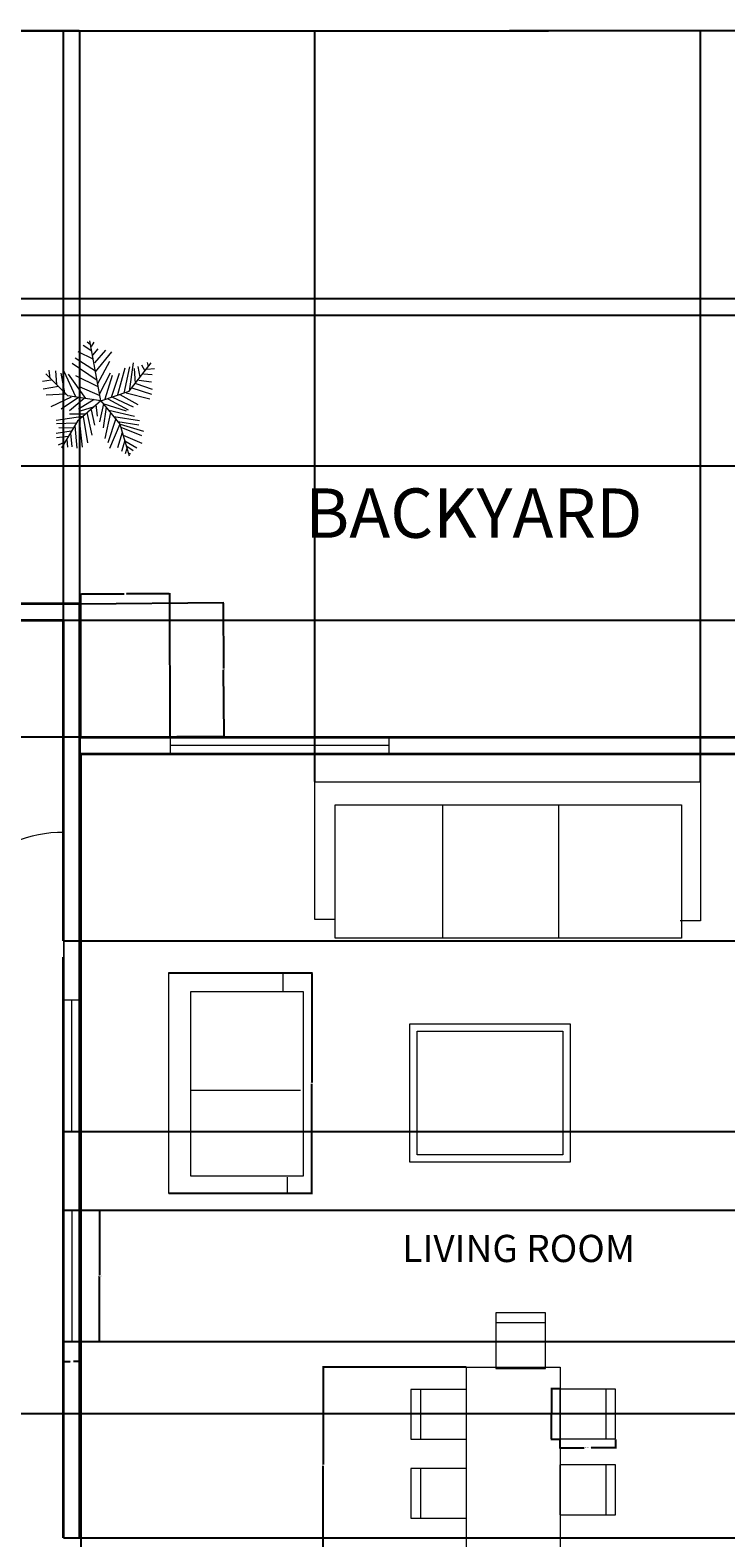
# Model space of a CAD drawing. Units: inches. Extents: x -86 to 773, y -188 to 560.
# Tile 3 of 6: x 201 to 392, y 147 to 560. Entities that reach past the tile are written whole.
import ezdxf

# ---------------------------------------------------------------- set-up
doc = ezdxf.new("R2010")
doc.units = ezdxf.units.IN
doc.header["$MEASUREMENT"] = 0
for name, color, linetype, lineweight in [('A-ANNO-DIMS', 2, 'Continuous', 18), ('A-AREA-IDEN', 7, 'Continuous', 25), ('A-DOOR', 7, 'Continuous', 18), ('A-FURN', 8, 'Continuous', 18), ('A-GLAZ', 7, 'Continuous', 18), ('A-WALL', 7, 'Continuous', 35), ('C-PROP', 7, 'Continuous', 25), ('L-PLNT-TREE', 8, 'Continuous', 9)]:
    doc.layers.add(name, color=color, linetype=linetype, lineweight=lineweight)
doc.styles.get("Standard").update_dxf_attribs({"font": 'arial.ttf'})
doc.dimstyles.get("Standard").update_dxf_attribs({"dimtxt": 0.18, "dimasz": 0.18, "dimexe": 0.18, "dimexo": 0.0625, "dimgap": 0.09, "dimtad": 0, "dimtih": 1, "dimtoh": 1, "dimdec": 4, "dimzin": 0, "dimdsep": 46, "dimtxsty": 'Standard', "dimcen": 0.09, "dimadec": 0, "dimazin": 0, "dimtfac": 1, "dimtdec": 4, "dimtofl": 0, "dimtmove": 0, "dimatfit": 3, "dimfxl": 1, "dimtolj": 1, "dimtzin": 0, "dimarcsym": 0})

# ---------------------------------------------------------------- blocks, each defined once
blk = doc.blocks.new('Trees - Metric')
for p, q in [((-185.1152, 1008.5578), (-553.1612, 1185.4942)), ((-221.9198, 1197.3052), (-433.5526, 1338.8594)), ((-258.7244, 1362.456), (-332.3336, 1421.4348)), ((0, 0), (-266.7, 1447.8)), ((-231.1146, 1315.2628), (-166.7002, 1421.4348)), ((-194.31, 1102.9442), (-65.4812, 1256.284)), ((-148.3106, 914.1968), (118.5418, 1220.9018)), ((-129.8956, 701.8528), (265.7602, 1185.4942)), ((-1234.059, 536.7274), (-1252.4486, 737.2604)), ((-93.091, 489.5342), (-700.3796, 902.3858)), ((-129.8956, 713.6638), (-626.7704, 1032.1544)), ((-74.7014, 418.7444), (219.7608, 961.39)), ((412.9786, 147.447), (587.8068, 796.2392)), ((560.197, 182.8292), (698.2206, 819.8358)), ((685.8, 228.6), (1219.2, 914.4)), ((689.0258, 230.0224), (790.2448, 914.1968)), ((808.6344, 784.4282), (827.0494, 418.7444)), ((891.4384, 831.6214), (946.658, 572.1096)), ((983.4626, 867.0036), (1066.2666, 725.4494)), ((1112.2914, 760.8316), (1296.3144, 784.4282)), ((1121.4862, 925.9824), (1149.0706, 831.6214)), ((-1206.4492, 501.3198), (-1418.082, 465.9376)), ((-800.1, 114.3), (-1333.5, 647.7)), ((-1105.2302, 725.4494), (-1077.6458, 395.1732)), ((-976.4268, 666.4706), (-884.4026, 194.6402)), ((-902.8176, 713.6638), (-617.5756, 100.2538)), ((-369.1382, 53.086), (-783.1836, 642.874)), ((-617.5756, 607.4918), (-74.7014, 347.98)), ((-28.6766, 171.0436), (228.9556, 678.2816)), ((100.1268, 41.275), (284.1498, 619.2774)), ((256.5654, 88.4682), (449.7832, 666.4706)), ((845.439, 418.7444), (1241.0948, 277.1902)), ((919.0482, 501.3198), (1222.6798, 454.152)), ((1029.462, 654.685), (1241.0948, 631.0884)), ((-1031.621, 347.98), (-1399.667, 277.1902)), ((-847.598, 159.2326), (-1326.0578, 135.636)), ((-718.7946, 88.4682), (-1215.644, -147.447)), ((-543.9664, 76.6572), (-967.2066, -206.4512)), ((0, 0), (-800.1, 114.3)), ((-405.9428, 53.086), (-764.794, -241.8334)), ((0, 0), (-571.5, -495.3)), ((-166.7002, 29.4894), (-543.9664, -206.4512)), ((-525.5514, 347.98), (-28.6766, 123.8504)), ((0, 0), (685.8, 228.6)), ((0, 0), (457.2, -571.5)), ((164.5412, 41.275), (661.416, -218.2368)), ((284.1498, 88.4682), (781.0246, -147.447)), ((458.978, 147.447), (891.4384, -88.4682)), ((615.4166, 194.6402), (1185.8752, 41.275)), ((753.4148, 312.5978), (1222.6798, 159.2326)), ((-387.5278, -324.4088), (-764.794, -324.4088)), ((-166.7002, -147.447), (-507.1618, -253.619)), ((-341.5284, -289.0012), (-221.9198, -831.6214)), ((-240.3094, -218.2368), (-157.5054, -595.7062)), ((-120.7008, -88.4682), (-93.091, -371.5766)), ((63.3222, -76.6826), (-37.8714, -513.1308)), ((44.9326, -64.897), (615.4166, -241.8334)), ((127.7366, -159.258), (54.1274, -654.685)), ((228.9556, -289.0012), (90.932, -914.1968)), ((192.151, -230.0224), (817.8292, -371.5766)), ((-442.7474, -383.3876), (-1086.8406, -477.7486)), ((-617.5756, -548.5384), (-1077.6458, -560.324)), ((-681.9646, -666.496), (-1022.4262, -654.685)), ((-571.5, -495.3), (-952.5, -1143)), ((-635.9652, -607.5172), (-580.771, -1150.1374)), ((-525.5514, -465.963), (-451.9422, -1126.5408)), ((-433.5526, -383.3876), (-323.1134, -1020.3688)), ((357.759, -430.5554), (164.5412, -1020.3688)), ((458.978, -572.1096), (210.5406, -1161.923)), ((311.7596, -383.3876), (937.4378, -477.7486)), ((412.9786, -501.3452), (919.0482, -583.9206)), ((457.2, -571.5), (685.8, -1333.5)), ((468.1982, -572.1096), (1029.462, -737.2604)), ((486.5878, -642.8994), (983.4626, -843.4324)), ((-718.7946, -737.2604), (-1086.8406, -796.2392)), ((-783.1836, -867.029), (-1077.6458, -902.4112)), ((-875.2078, -1008.5832), (-1040.8412, -1079.3476)), ((-829.2084, -937.7934), (-810.7934, -1126.5408)), ((-737.1842, -784.4536), (-709.5744, -1114.7298)), ((514.1976, -772.6426), (403.7838, -1138.3264)), ((578.612, -961.39), (495.7826, -1232.7128)), ((541.8074, -831.6214), (992.6574, -1032.1544)), ((578.612, -973.1756), (873.0488, -1138.3264)), ((624.6114, -1161.923), (587.8068, -1291.6916)), ((624.6114, -1102.9442), (781.0246, -1209.1162)), ((679.8056, -1268.095), (716.6102, -1291.6916))]:
    blk.add_line(p, q)
blk = doc.blocks.new('WIN-60-W4_5')
for p, q in [((0, 4.5), (0, 0)), ((60, 4.5), (60, 0)), ((60, 2.25), (0, 2.25))]:
    blk.add_line(p, q)
blk = doc.blocks.new('WIN-36-W4_5')
for p, q in [((0, 36), (4.5, 36)), ((2.25, 36), (2.25, 0)), ((0, 0), (4.5, 0))]:
    blk.add_line(p, q)
blk = doc.blocks.new('DINING-CHAIR')
blk.add_line((0, 12.55), (13.8, 12.55))
blk.add_lwpolyline([(0.02, 0), (13.65, 0), (13.65, 15.22), (0.02, 15.22)], close=True)
blk = doc.blocks.new('*D19')
at = {"layer": 'A-ANNO-DIMS', "color": 0, "lineweight": -2, "transparency": 16777216}
for p, q in [((346.32, 174.18), (346.32, 171.78)), ((361.54, 174.18), (361.54, 171.78)), ((346.5, 171.96), (352.98, 171.96)), ((361.36, 171.96), (354.89, 171.96))]:
    blk.add_line(p, q, dxfattribs=at)
at = {"layer": 'A-ANNO-DIMS', "color": 0, "transparency": 16777216}
for points in [[(346.5, 171.99), (346.5, 171.93), (346.32, 171.96)], [(361.36, 171.99), (361.36, 171.93), (361.54, 171.96)]]:
    blk.add_solid(points, dxfattribs=at)
at = {"layer": 'Defpoints', "color": 0, "transparency": 16777216}
for p in [(346.32, 174.25), (361.54, 174.25), (361.54, 171.96)]:
    blk.add_point(p, dxfattribs=at)
at = {"layer": 'A-ANNO-DIMS', "color": 0, "transparency": 16777216, "insert": (353.93, 171.96), "char_height": 0.18, "attachment_point": 5}
blk.add_mtext('\\A1;CHAIR 15 TYP.', dxfattribs=at)
blk = doc.blocks.new('*D20')
at = {"layer": 'A-ANNO-DIMS', "color": 0, "lineweight": -2, "transparency": 16777216}
for p, q in [((346.26, 188.05), (343.86, 188.05)), ((344.04, 187.87), (344.04, 181.33)), ((344.04, 174.43), (344.04, 180.97)), ((346.26, 174.25), (343.86, 174.25))]:
    blk.add_line(p, q, dxfattribs=at)
at = {"layer": 'A-ANNO-DIMS', "color": 0, "transparency": 16777216}
for points in [[(344.01, 187.87), (344.07, 187.87), (344.04, 188.05)], [(344.01, 174.43), (344.07, 174.43), (344.04, 174.25)]]:
    blk.add_solid(points, dxfattribs=at)
at = {"layer": 'Defpoints', "color": 0, "transparency": 16777216}
for p in [(346.32, 188.05), (344.04, 174.25), (346.32, 174.25)]:
    blk.add_point(p, dxfattribs=at)
at = {"layer": 'A-ANNO-DIMS', "color": 0, "transparency": 16777216, "insert": (344.04, 181.15), "char_height": 0.18, "attachment_point": 5}
blk.add_mtext('\\A1;14 TYP.', dxfattribs=at)
blk = doc.blocks.new('*D37')
at = {"layer": 'A-ANNO-DIMS', "color": 0, "lineweight": -2, "transparency": 16777216}
for p, q in [((214.83, 237.01), (220.34, 237.01)), ((220.16, 236.83), (220.16, 219.19)), ((220.16, 201.19), (220.16, 218.82)), ((214.83, 201.01), (220.34, 201.01))]:
    blk.add_line(p, q, dxfattribs=at)
at = {"layer": 'A-ANNO-DIMS', "color": 0, "transparency": 16777216}
for points in [[(220.13, 236.83), (220.19, 236.83), (220.16, 237.01)], [(220.13, 201.19), (220.19, 201.19), (220.16, 201.01)]]:
    blk.add_solid(points, dxfattribs=at)
at = {"layer": 'Defpoints', "color": 0, "transparency": 16777216}
for p in [(214.76, 237.01), (220.16, 237.01), (214.76, 201.01)]:
    blk.add_point(p, dxfattribs=at)
at = {"layer": 'A-ANNO-DIMS', "color": 0, "transparency": 16777216, "insert": (220.16, 219.01), "char_height": 0.18, "attachment_point": 5}
blk.add_mtext('\\A1;WINDOW 36 TYP.', dxfattribs=at)
blk = doc.blocks.new('*D38')
at = {"layer": 'A-ANNO-DIMS', "color": 0, "lineweight": -2, "transparency": 16777216}
for p, q in [((210.26, 200.94), (210.26, 195.43)), ((214.76, 200.94), (214.76, 195.43)), ((210.44, 195.61), (212.06, 195.61)), ((214.58, 195.61), (212.97, 195.61))]:
    blk.add_line(p, q, dxfattribs=at)
at = {"layer": 'A-ANNO-DIMS', "color": 0, "transparency": 16777216}
for points in [[(210.44, 195.64), (210.44, 195.58), (210.26, 195.61)], [(214.58, 195.64), (214.58, 195.58), (214.76, 195.61)]]:
    blk.add_solid(points, dxfattribs=at)
at = {"layer": 'Defpoints', "color": 0, "transparency": 16777216}
for p in [(210.26, 201.01), (214.76, 201.01), (214.76, 195.61)]:
    blk.add_point(p, dxfattribs=at)
at = {"layer": 'A-ANNO-DIMS', "color": 0, "transparency": 16777216, "insert": (212.51, 195.61), "char_height": 0.18, "attachment_point": 5}
blk.add_mtext('\\A1;5 TYP.', dxfattribs=at)
blk = doc.blocks.new('*D45')
at = {"layer": 'A-ANNO-DIMS', "color": 0, "lineweight": -2, "transparency": 16777216}
for p, q in [((-46.55, 486.72), (-46.55, 560.19)), ((-46.37, 560.01), (343.16, 560.01)), ((733.27, 560.01), (343.74, 560.01)), ((733.45, 486.72), (733.45, 560.19))]:
    blk.add_line(p, q, dxfattribs=at)
at = {"layer": 'A-ANNO-DIMS', "color": 0, "transparency": 16777216}
for points in [[(-46.37, 560.04), (-46.37, 559.98), (-46.55, 560.01)], [(733.27, 560.04), (733.27, 559.98), (733.45, 560.01)]]:
    blk.add_solid(points, dxfattribs=at)
at = {"layer": 'Defpoints', "color": 0, "transparency": 16777216}
for p in [(733.45, 560.01), (-46.55, 486.66), (733.45, 486.66)]:
    blk.add_point(p, dxfattribs=at)
at = {"layer": 'A-ANNO-DIMS', "color": 0, "transparency": 16777216, "insert": (343.45, 560.01), "char_height": 0.18, "attachment_point": 5}
blk.add_mtext('\\A1;780', dxfattribs=at)
blk = doc.blocks.new('*D55')
at = {"layer": 'A-ANNO-DIMS', "color": 0, "lineweight": -2, "transparency": 16777216}
for p, q in [((450.97, 440.74), (-85.98, 440.74)), ((-85.8, 440.56), (-85.8, 403.81)), ((-85.8, 366.7), (-85.8, 403.45)), ((450.97, 366.52), (-85.98, 366.52))]:
    blk.add_line(p, q, dxfattribs=at)
at = {"layer": 'A-ANNO-DIMS', "color": 0, "transparency": 16777216}
for points in [[(-85.83, 440.56), (-85.77, 440.56), (-85.8, 440.74)], [(-85.83, 366.7), (-85.77, 366.7), (-85.8, 366.52)]]:
    blk.add_solid(points, dxfattribs=at)
at = {"layer": 'Defpoints', "color": 0, "transparency": 16777216}
for p in [(451.03, 440.74), (-85.8, 366.52), (451.03, 366.52)]:
    blk.add_point(p, dxfattribs=at)
at = {"layer": 'A-ANNO-DIMS', "color": 0, "transparency": 16777216, "insert": (-85.8, 403.63), "char_height": 0.18, "attachment_point": 5}
blk.add_mtext('\\A1;74.22', dxfattribs=at)
blk = doc.blocks.new('*D56')
at = {"layer": 'A-ANNO-DIMS', "color": 0, "lineweight": -2, "transparency": 16777216}
for p, q in [((13.45, 403.19), (13.45, 560.19)), ((13.63, 560.01), (113.71, 560.01)), ((214.57, 560.01), (114.5, 560.01)), ((214.75, 403.19), (214.75, 560.19))]:
    blk.add_line(p, q, dxfattribs=at)
at = {"layer": 'A-ANNO-DIMS', "color": 0, "transparency": 16777216}
for points in [[(13.63, 560.04), (13.63, 559.98), (13.45, 560.01)], [(214.57, 560.04), (214.57, 559.98), (214.75, 560.01)]]:
    blk.add_solid(points, dxfattribs=at)
at = {"layer": 'Defpoints', "color": 0, "transparency": 16777216}
for p in [(214.75, 560.01), (13.45, 403.12), (214.75, 403.12)]:
    blk.add_point(p, dxfattribs=at)
at = {"layer": 'A-ANNO-DIMS', "color": 0, "transparency": 16777216, "insert": (114.1, 560.01), "char_height": 0.18, "attachment_point": 5}
blk.add_mtext('\\A1;201.3', dxfattribs=at)
blk = doc.blocks.new('*D58')
at = {"layer": 'A-ANNO-DIMS', "color": 0, "lineweight": -2, "transparency": 16777216}
for p, q in [((136.03, 398.69), (136.03, 560.19)), ((136.21, 560.01), (172.75, 560.01)), ((210.07, 560.01), (173.53, 560.01)), ((210.25, 398.69), (210.25, 560.19))]:
    blk.add_line(p, q, dxfattribs=at)
at = {"layer": 'A-ANNO-DIMS', "color": 0, "transparency": 16777216}
for points in [[(136.21, 560.04), (136.21, 559.98), (136.03, 560.01)], [(210.07, 560.04), (210.07, 559.98), (210.25, 560.01)]]:
    blk.add_solid(points, dxfattribs=at)
at = {"layer": 'Defpoints', "color": 0, "transparency": 16777216}
for p in [(210.25, 560.01), (136.03, 398.62), (210.25, 398.62)]:
    blk.add_point(p, dxfattribs=at)
at = {"layer": 'A-ANNO-DIMS', "color": 0, "transparency": 16777216, "insert": (173.14, 560.01), "char_height": 0.18, "attachment_point": 5}
blk.add_mtext('\\A1;74.22', dxfattribs=at)
blk = doc.blocks.new('*D61')
at = {"layer": 'A-ANNO-DIMS', "color": 0, "lineweight": -2, "transparency": 16777216}
for p, q in [((210.31, 398.62), (772.88, 398.62)), ((772.7, 398.44), (772.7, 354.88)), ((772.7, 310.95), (772.7, 354.52)), ((210.31, 310.77), (772.88, 310.77))]:
    blk.add_line(p, q, dxfattribs=at)
at = {"layer": 'A-ANNO-DIMS', "color": 0, "transparency": 16777216}
for points in [[(772.67, 398.44), (772.73, 398.44), (772.7, 398.62)], [(772.67, 310.95), (772.73, 310.95), (772.7, 310.77)]]:
    blk.add_solid(points, dxfattribs=at)
at = {"layer": 'Defpoints', "color": 0, "transparency": 16777216}
for p in [(210.25, 398.62), (210.25, 310.77), (772.7, 310.77)]:
    blk.add_point(p, dxfattribs=at)
at = {"layer": 'A-ANNO-DIMS', "color": 0, "transparency": 16777216, "insert": (772.7, 354.7), "char_height": 0.18, "attachment_point": 5}
blk.add_mtext('\\A1;87.85', dxfattribs=at)
blk = doc.blocks.new('*D62')
at = {"layer": 'A-ANNO-DIMS', "color": 0, "lineweight": -2, "transparency": 16777216}
for p, q in [((210.33, 201.01), (772.88, 201.01)), ((772.7, 200.83), (772.7, 174.33)), ((772.7, 147.46), (772.7, 173.96)), ((210.31, 147.28), (772.88, 147.28))]:
    blk.add_line(p, q, dxfattribs=at)
at = {"layer": 'A-ANNO-DIMS', "color": 0, "transparency": 16777216}
for points in [[(772.67, 200.83), (772.73, 200.83), (772.7, 201.01)], [(772.67, 147.46), (772.73, 147.46), (772.7, 147.28)]]:
    blk.add_solid(points, dxfattribs=at)
at = {"layer": 'Defpoints', "color": 0, "transparency": 16777216}
for p in [(210.26, 201.01), (210.25, 147.28), (772.7, 147.28)]:
    blk.add_point(p, dxfattribs=at)
at = {"layer": 'A-ANNO-DIMS', "color": 0, "transparency": 16777216, "insert": (772.7, 174.14), "char_height": 0.18, "attachment_point": 5}
blk.add_mtext('\\A1;53.72', dxfattribs=at)
blk = doc.blocks.new('*D65')
at = {"layer": 'A-ANNO-DIMS', "color": 0, "lineweight": -2, "transparency": 16777216}
for p, q in [((446.53, 366.45), (446.53, -187.76)), ((215.06, 361.95), (215.06, -187.76)), ((215.24, -187.58), (330.33, -187.58)), ((446.35, -187.58), (331.26, -187.58))]:
    blk.add_line(p, q, dxfattribs=at)
at = {"layer": 'A-ANNO-DIMS', "color": 0, "transparency": 16777216}
for points in [[(215.24, -187.55), (215.24, -187.61), (215.06, -187.58)], [(446.35, -187.55), (446.35, -187.61), (446.53, -187.58)]]:
    blk.add_solid(points, dxfattribs=at)
at = {"layer": 'Defpoints', "color": 0, "transparency": 16777216}
for p in [(446.53, 366.52), (215.06, 362.02), (446.53, -187.58)]:
    blk.add_point(p, dxfattribs=at)
at = {"layer": 'A-ANNO-DIMS', "color": 0, "transparency": 16777216, "insert": (330.8, -187.58), "char_height": 0.18, "attachment_point": 5}
blk.add_mtext('\\A1;231.47', dxfattribs=at)
blk = doc.blocks.new('*D73')
at = {"layer": 'A-ANNO-DIMS', "color": 0, "lineweight": -2, "transparency": 16777216}
for p, q in [((577.4, 181.27), (-85.98, 181.27)), ((-85.8, 181.09), (-85.8, 145.29)), ((-85.8, 109.12), (-85.8, 144.92)), ((577.4, 108.94), (-85.98, 108.94))]:
    blk.add_line(p, q, dxfattribs=at)
at = {"layer": 'A-ANNO-DIMS', "color": 0, "transparency": 16777216}
for points in [[(-85.83, 181.09), (-85.77, 181.09), (-85.8, 181.27)], [(-85.83, 109.12), (-85.77, 109.12), (-85.8, 108.94)]]:
    blk.add_solid(points, dxfattribs=at)
at = {"layer": 'Defpoints', "color": 0, "transparency": 16777216}
for p in [(-85.8, 181.27), (577.46, 181.27), (577.46, 108.94)]:
    blk.add_point(p, dxfattribs=at)
at = {"layer": 'A-ANNO-DIMS', "color": 0, "transparency": 16777216, "insert": (-85.8, 145.11), "char_height": 0.18, "attachment_point": 5}
blk.add_mtext('\\A1;72.33', dxfattribs=at)
blk = doc.blocks.new('*D75')
at = {"layer": 'A-ANNO-DIMS', "color": 0, "lineweight": -2, "transparency": 16777216}
for p, q in [((279.19, 354.43), (279.19, 560.19)), ((279.37, 560.01), (331.56, 560.01)), ((384.66, 560.01), (332.47, 560.01)), ((384.84, 354.43), (384.84, 560.19))]:
    blk.add_line(p, q, dxfattribs=at)
at = {"layer": 'A-ANNO-DIMS', "color": 0, "transparency": 16777216}
for points in [[(279.37, 560.04), (279.37, 559.98), (279.19, 560.01)], [(384.66, 560.04), (384.66, 559.98), (384.84, 560.01)]]:
    blk.add_solid(points, dxfattribs=at)
at = {"layer": 'Defpoints', "color": 0, "transparency": 16777216}
for p in [(384.84, 560.01), (279.19, 354.36), (384.84, 354.36)]:
    blk.add_point(p, dxfattribs=at)
at = {"layer": 'A-ANNO-DIMS', "color": 0, "transparency": 16777216, "insert": (332.02, 560.01), "char_height": 0.18, "attachment_point": 5}
blk.add_mtext('\\A1;105.65', dxfattribs=at)
blk = doc.blocks.new('*D76')
at = {"layer": 'A-ANNO-DIMS', "color": 0, "lineweight": -2, "transparency": 16777216}
for p, q in [((239.14, 301.98), (278.5, 301.98)), ((278.32, 301.8), (278.32, 272.01)), ((278.32, 241.85), (278.32, 271.65)), ((239.14, 241.67), (278.5, 241.67))]:
    blk.add_line(p, q, dxfattribs=at)
at = {"layer": 'A-ANNO-DIMS', "color": 0, "transparency": 16777216}
for points in [[(278.29, 301.8), (278.35, 301.8), (278.32, 301.98)], [(278.29, 241.85), (278.35, 241.85), (278.32, 241.67)]]:
    blk.add_solid(points, dxfattribs=at)
at = {"layer": 'Defpoints', "color": 0, "transparency": 16777216}
for p in [(239.07, 301.98), (239.07, 241.67), (278.32, 241.67)]:
    blk.add_point(p, dxfattribs=at)
at = {"layer": 'A-ANNO-DIMS', "color": 0, "transparency": 16777216, "insert": (278.32, 271.83), "char_height": 0.18, "attachment_point": 5}
blk.add_mtext('\\A1;60.32', dxfattribs=at)
blk = doc.blocks.new('*D78')
at = {"layer": 'A-ANNO-DIMS', "color": 0, "lineweight": -2, "transparency": 16777216}
for p, q in [((320.63, 194.07), (281.26, 194.07)), ((281.44, 193.89), (281.44, 167.41)), ((281.44, 140.57), (281.44, 167.05)), ((320.63, 140.39), (281.26, 140.39))]:
    blk.add_line(p, q, dxfattribs=at)
at = {"layer": 'A-ANNO-DIMS', "color": 0, "transparency": 16777216}
for points in [[(281.41, 193.89), (281.47, 193.89), (281.44, 194.07)], [(281.41, 140.57), (281.47, 140.57), (281.44, 140.39)]]:
    blk.add_solid(points, dxfattribs=at)
at = {"layer": 'Defpoints', "color": 0, "transparency": 16777216}
for p in [(281.44, 194.07), (320.69, 194.07), (320.69, 140.39)]:
    blk.add_point(p, dxfattribs=at)
at = {"layer": 'A-ANNO-DIMS', "color": 0, "transparency": 16777216, "insert": (281.44, 167.23), "char_height": 0.18, "attachment_point": 5}
blk.add_mtext('\\A1;53.68', dxfattribs=at)
blk = doc.blocks.new('*D79')
at = {"layer": 'A-ANNO-DIMS', "color": 0, "lineweight": -2, "transparency": 16777216}
for p, q in [((210.31, 258.61), (772.88, 258.61)), ((772.7, 258.43), (772.7, 247.99)), ((772.7, 237.19), (772.7, 247.63)), ((210.33, 237.01), (772.88, 237.01))]:
    blk.add_line(p, q, dxfattribs=at)
at = {"layer": 'A-ANNO-DIMS', "color": 0, "transparency": 16777216}
for points in [[(772.67, 258.43), (772.73, 258.43), (772.7, 258.61)], [(772.67, 237.19), (772.73, 237.19), (772.7, 237.01)]]:
    blk.add_solid(points, dxfattribs=at)
at = {"layer": 'Defpoints', "color": 0, "transparency": 16777216}
for p in [(210.24, 258.61), (210.26, 237.01), (772.7, 237.01)]:
    blk.add_point(p, dxfattribs=at)
at = {"layer": 'A-ANNO-DIMS', "color": 0, "transparency": 16777216, "insert": (772.7, 247.81), "char_height": 0.18, "attachment_point": 5}
blk.add_mtext('\\A1;21.604', dxfattribs=at)
blk = doc.blocks.new('*D81')
at = {"layer": 'A-ANNO-DIMS', "color": 0, "lineweight": -2, "transparency": 16777216}
for p, q in [((214.81, 403.12), (254.18, 403.46)), ((254, 403.28), (254.15, 385.33)), ((254.31, 367.03), (254.16, 384.97)), ((215.12, 366.52), (254.49, 366.85))]:
    blk.add_line(p, q, dxfattribs=at)
at = {"layer": 'A-ANNO-DIMS', "color": 0, "transparency": 16777216}
for points in [[(254.03, 403.28), (253.97, 403.27), (254, 403.46)], [(254.34, 367.03), (254.28, 367.03), (254.31, 366.85)]]:
    blk.add_solid(points, dxfattribs=at)
at = {"layer": 'Defpoints', "color": 0, "transparency": 16777216}
for p in [(214.75, 403.12), (215.06, 366.52), (254.31, 366.85)]:
    blk.add_point(p, dxfattribs=at)
at = {"layer": 'A-ANNO-DIMS', "color": 0, "transparency": 16777216, "insert": (254.16, 385.15), "char_height": 0.18, "attachment_point": 5}
blk.add_mtext('\\A1;36.61', dxfattribs=at)
blk = doc.blocks.new('*D87')
at = {"layer": 'A-ANNO-DIMS', "color": 0, "lineweight": -2, "transparency": 16777216}
for p, q in [((215.06, 366.58), (215.04, 405.95)), ((215.22, 405.77), (226.91, 405.77)), ((239.26, 405.78), (227.56, 405.77)), ((239.46, 366.59), (239.44, 405.96))]:
    blk.add_line(p, q, dxfattribs=at)
at = {"layer": 'A-ANNO-DIMS', "color": 0, "transparency": 16777216}
for points in [[(215.22, 405.8), (215.22, 405.74), (215.04, 405.77)], [(239.26, 405.81), (239.26, 405.75), (239.44, 405.78)]]:
    blk.add_solid(points, dxfattribs=at)
at = {"layer": 'Defpoints', "color": 0, "transparency": 16777216}
for p in [(239.44, 405.78), (215.06, 366.52), (239.46, 366.53)]:
    blk.add_point(p, dxfattribs=at)
at = {"layer": 'A-ANNO-DIMS', "color": 0, "transparency": 16777216, "insert": (227.24, 405.77), "char_height": 0.18, "attachment_point": 5}
blk.add_mtext('\\A1;24.4', dxfattribs=at)

msp = doc.modelspace()

# ---------------------------------------------------------------- linework, layer by layer
at = {"layer": 'A-DOOR'}
for p, q in [((210.3869, 340.4977), (210.3869, 304.4977)), ((210.3349, 275.2294), (210.3349, 311.2294))]:
    msp.add_line(p, q, dxfattribs=at)
msp.add_arc((210.3869, 304.4977), 36, 90, 177.176183, dxfattribs=at)
at = {"layer": 'A-FURN'}
for p, q in [((314.142, 348.0153), (314.142, 311.5084)), ((345.9171, 348.0153), (345.9171, 311.5084)), ((245.0311, 269.8429), (275.2174, 269.8429))]:
    msp.add_line(p, q, dxfattribs=at)
for points in [[(284.75, 316.667), (279.1893, 316.667), (279.1893, 354.3643), (384.8416, 354.3643), (384.8416, 316.2702), (379.281, 316.2702)], [(270.4512, 296.8263), (270.4512, 301.9849), (239.0733, 301.9849), (239.0733, 241.6692), (271.6428, 241.6692), (271.6428, 246.0341)]]:
    msp.add_lwpolyline(points, dxfattribs=at)
for points in [[(284.75, 348.0153), (379.6782, 348.0153), (379.6782, 311.5084), (284.75, 311.5084)], [(276.0118, 296.8263), (245.0311, 296.8263), (245.0311, 246.4309), (276.0118, 246.4309)], [(305.2234, 288.0373), (349.12, 288.0373), (349.12, 250.1624), (305.2234, 250.1624)], [(307.2234, 286.0373), (347.12, 286.0373), (347.12, 252.1624), (307.2234, 252.1624)], [(320.6933, 194.0682), (346.3535, 194.0682), (346.3535, 140.3929), (320.6933, 140.3929)]]:
    msp.add_lwpolyline(points, close=True, dxfattribs=at)
at = {"layer": 'A-WALL'}
for p, q in [((13.4515, 403.1228), (214.7515, 403.1228)), ((214.7515, 147.2828), (214.7515, 403.1228)), ((136.0315, 398.6228), (210.2515, 398.6228)), ((210.2515, 310.7712), (210.2515, 398.6228)), ((210.2515, 147.2828), (210.2515, 306.2712))]:
    msp.add_line(p, q, dxfattribs=at)
for points in [[(215.0615, 366.5167), (451.0315, 366.5167)], [(215.0615, 362.0167), (405.4862, 362.0167)]]:
    msp.add_lwpolyline(points, dxfattribs=at)
at = {"layer": 'C-PROP'}
for p, q in [((-46.5485, 486.6589), (733.4515, 486.6589)), ((-42.0485, 482.1589), (728.9515, 482.1589))]:
    msp.add_line(p, q, dxfattribs=at)

# ---------------------------------------------------------------- block references
at = {"layer": 'A-FURN'}
msp.add_blockref('DINING-CHAIR', (328.697, 193.668), dxfattribs=at)
for p, rotation in [((320.7221, 174.246), 89.9999999999998), ((346.3239, 188.0478), 270), ((320.7221, 152.664), 89.99999999999969), ((346.3239, 167.2592), 270.0000000000002)]:
    msp.add_blockref('DINING-CHAIR', p, dxfattribs=dict(at, rotation=rotation))
at = {"layer": 'A-GLAZ'}
for name, p in [('WIN-60-W4_5', (239.463, 362.032)), ('WIN-36-W4_5', (210.2446, 258.6103)), ('WIN-36-W4_5', (210.265, 201.006))]:
    msp.add_blockref(name, p, dxfattribs=at)
at = {"layer": 'L-PLNT-TREE', "xscale": 0.0112992005060107, "yscale": 0.0112992005060107, "zscale": 0.0112992005060107}
msp.add_blockref('Trees - Metric', (220.5253, 458.7065), dxfattribs=at)

# ---------------------------------------------------------------- texts
at = {"layer": 'A-AREA-IDEN'}
for s, height, p in [('BACKYARD', 13.52574, (276.4717, 421.1552)), ('LIVING ROOM', 7.452962, (303.1214, 222.8126))]:
    msp.add_text(s, height=height, dxfattribs=at).set_placement(p)

# ---------------------------------------------------------------- dimensions: what is measured, and where the dimension line sits
at = {"layer": 'A-ANNO-DIMS'}
for base, p1, p2, override, picture, middle in [((733.4515, 560.0063), (-46.5485, 486.6589), (733.4515, 486.6589), {"dimdec": 0, "dimlfac": 1, "dimrnd": 0, "dimzin": 0, "dimdsep": 46, "dimlunit": 2}, '*D45', (343.4515, 560.0063)), ((214.7515, 560.0063), (13.4515, 403.1228), (214.7515, 403.1228), {"dimdec": 1, "dimlfac": 1, "dimrnd": 0, "dimzin": 0, "dimdsep": 46, "dimlunit": 2}, '*D56', (114.1015, 560.0063)), ((210.2515, 560.0063), (136.0315, 398.6228), (210.2515, 398.6228), {"dimdec": 2, "dimlfac": 1, "dimrnd": 0, "dimzin": 0, "dimdsep": 46, "dimlunit": 2}, '*D58', (173.1415, 560.0063)), ((384.8416, 560.0063), (279.1893, 354.3643), (384.8416, 354.3643), {"dimdec": 2, "dimlfac": 1, "dimrnd": 0, "dimzin": 0, "dimdsep": 46, "dimlunit": 2}, '*D75', (332.0155, 560.0063)), ((446.5315, -187.578), (215.0615, 362.0167), (446.5315, 366.5167), {"dimdec": 2, "dimlfac": 1, "dimrnd": 0, "dimzin": 0, "dimdsep": 46, "dimlunit": 2}, '*D65', (330.7965, -187.578))]:
    dim = msp.add_linear_dim(base=base, p1=p1, p2=p2, dimstyle='Standard', override=override, dxfattribs=at)
    dim.commit()
    dim.dimension.update_dxf_attribs({"geometry": picture, "text_midpoint": middle})
for base, p1, p2, angle, override, picture, middle in [((-85.7985, 366.5167), (451.0315, 440.7367), (451.0315, 366.5167), 90, {"dimdec": 2, "dimlfac": 1, "dimrnd": 0, "dimzin": 0, "dimdsep": 46, "dimlunit": 2}, '*D55', (-85.7985, 403.6267)), ((239.4388, 405.782), (215.0615, 366.5167), (239.4634, 366.532), 0.035999, {"dimdec": 1, "dimlfac": 1, "dimrnd": 0, "dimzin": 0, "dimdsep": 46, "dimlunit": 2}, '*D87', (227.2378, 405.7743)), ((254.3101, 366.849), (214.7515, 403.1228), (215.0615, 366.5167), 270.485172, {"dimdec": 2, "dimlfac": 1, "dimrnd": 0, "dimzin": 0, "dimdsep": 46, "dimlunit": 2}, '*D81', (254.1551, 385.1521)), ((772.7015, 310.7712), (210.2515, 398.6228), (210.2515, 310.7712), 90, {"dimdec": 2, "dimlfac": 1, "dimrnd": 0, "dimzin": 0, "dimdsep": 46, "dimlunit": 2}, '*D61', (772.7015, 354.697)), ((278.3233, 241.6692), (239.0733, 301.9849), (239.0733, 241.6692), 270, {"dimdec": 2, "dimlfac": 1, "dimrnd": 0, "dimzin": 0, "dimdsep": 46, "dimlunit": 2}, '*D76', (278.3233, 271.827)), ((772.7015, 237.0056), (210.2444, 258.61), (210.2647, 237.0056), 90, {"dimdec": 3, "dimlfac": 1, "dimrnd": 0, "dimzin": 0, "dimdsep": 46, "dimlunit": 2}, '*D79', (772.7015, 247.8078)), ((772.7015, 147.2828), (210.2647, 201.0056), (210.2515, 147.2828), 90, {"dimdec": 2, "dimlfac": 1, "dimrnd": 0, "dimzin": 0, "dimdsep": 46, "dimlunit": 2}, '*D62', (772.7015, 174.1442)), ((281.4433, 194.0682), (320.6933, 140.3929), (320.6933, 194.0682), 90, {"dimdec": 2, "dimlfac": 1, "dimrnd": 0, "dimzin": 0, "dimdsep": 46, "dimlunit": 2}, '*D78', (281.4433, 167.2305)), ((-85.7985, 181.2736), (577.46, 108.94), (577.46, 181.2736), 90, {"dimdec": 2, "dimlfac": 1, "dimrnd": 0, "dimzin": 0, "dimdsep": 46, "dimlunit": 2}, '*D73', (-85.7985, 145.1068))]:
    dim = msp.add_linear_dim(base=base, p1=p1, p2=p2, angle=angle, dimstyle='Standard', override=override, dxfattribs=at)
    dim.commit()
    dim.dimension.update_dxf_attribs({"geometry": picture, "text_midpoint": middle})
for base, p1, p2, angle, text, picture, middle in [((220.1647, 237.0056), (214.7647, 201.0056), (214.7647, 237.0056), 90, 'WINDOW <> TYP.', '*D37', (220.1647, 219.0056)), ((344.0403, 174.2464), (346.3235, 188.0474), (346.3235, 174.2464), 270, '<> TYP.', '*D20', (344.0403, 181.1469))]:
    dim = msp.add_linear_dim(base=base, p1=p1, p2=p2, angle=angle, text=text, dimstyle='Standard', override={"dimdec": 0, "dimlfac": 1, "dimrnd": 0, "dimzin": 0, "dimdsep": 46, "dimlunit": 2}, dxfattribs=at)
    dim.commit()
    dim.dimension.update_dxf_attribs({"geometry": picture, "text_midpoint": middle})
for base, p1, p2, text, picture, middle in [((214.7647399587, 195.6056477747), (210.2647399587, 201.0056477747), (214.7647399587, 201.0056477747), '<> TYP.', '*D38', (212.5147399587, 195.6056477747)), ((361.5448, 171.9632), (346.3235, 174.2464), (361.5448, 174.2464), 'CHAIR <> TYP.', '*D19', (353.9341, 171.9632))]:
    dim = msp.add_linear_dim(base=base, p1=p1, p2=p2, text=text, dimstyle='Standard', override={"dimdec": 0, "dimlfac": 1, "dimrnd": 0, "dimzin": 0, "dimdsep": 46, "dimlunit": 2}, dxfattribs=at)
    dim.commit()
    dim.dimension.update_dxf_attribs({"geometry": picture, "text_midpoint": middle})

doc.saveas('drawing.dxf')
